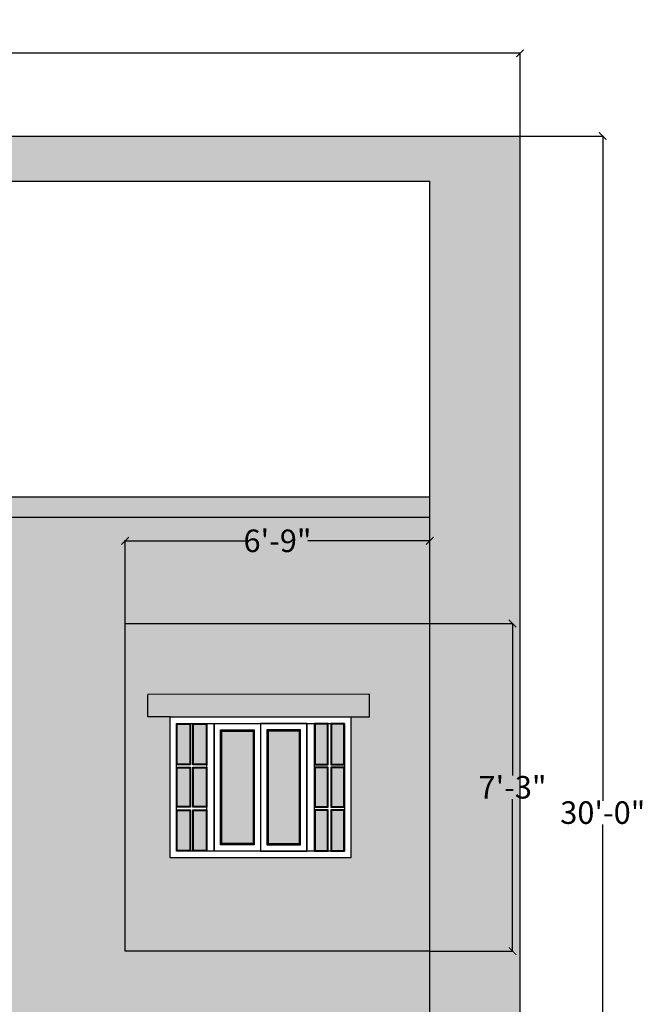
# Model space of a CAD drawing. Units: inches. Extents: x 528 to 2620, y -1066 to 798.
# Tile 41 of 41: x 2453 to 2620, y -891 to -629. Entities that reach past the tile are written whole.
import ezdxf

# ---------------------------------------------------------------- set-up
doc = ezdxf.new("R2010")
doc.units = ezdxf.units.IN
doc.header["$MEASUREMENT"] = 0
for name, color, linetype, lineweight in [('A-ANNO-DIMS', 2, 'Continuous', 18), ('A-ELEV', 7, 'Continuous', 25), ('A-ELEV-PATT', 8, 'Continuous', 13)]:
    doc.layers.add(name, color=color, linetype=linetype, lineweight=lineweight)
doc.styles.get("Standard").update_dxf_attribs({"font": 'arial.ttf'})
doc.dimstyles.get("Standard").update_dxf_attribs({"dimtxt": 6, "dimasz": 2, "dimexe": 0.18, "dimexo": 0.0625, "dimgap": 0.09, "dimtad": 0, "dimtih": 1, "dimtoh": 1, "dimdec": 1, "dimzin": 0, "dimdsep": 46, "dimlunit": 3, "dimtxsty": 'Standard', "dimblk": 'ARCHTICK', "dimcen": 0.09, "dimadec": 0, "dimazin": 0, "dimtfac": 1, "dimtdec": 1, "dimtofl": 0, "dimtmove": 0, "dimatfit": 3, "dimfxl": 1, "dimtolj": 1, "dimtzin": 0, "dimarcsym": 0})

# ---------------------------------------------------------------- blocks, each defined once
blk = doc.blocks.new('ww')
at = {"color": 0, "linetype": 'ByBlock'}
for p, q in [((30.67, -16.13), (126.65, -16.13)), ((30.67, -91.08), (30.67, -16.13)), ((34.01, -19.6), (123.32, -19.6)), ((34.01, -87.61), (34.01, -19.6)), ((34.01, -19.6), (49.87, -19.6)), ((34.01, -87.61), (34.01, -19.6)), ((50.03, -87.61), (50.03, -19.6)), ((54.03, -19.6), (54.03, -87.61)), ((103.29, -19.6), (103.29, -87.61)), ((107.29, -87.61), (107.29, -19.6)), ((123.32, -19.6), (123.32, -87.61)), ((126.65, -16.13), (126.65, -91.08)), ((123.32, -87.61), (34.01, -87.61)), ((126.65, -91.08), (30.67, -91.08))]:
    blk.add_line(p, q, dxfattribs=at)
at = {"color": 0, "linetype": 'ByBlock', "ltscale": 25}
for p, q in [((34.01, -41.58), (34.01, -19.6)), ((34.01, -19.6), (41.35, -19.6)), ((34.34, -41.23), (34.34, -19.95)), ((34.34, -19.95), (41.02, -19.95)), ((41.02, -19.95), (41.02, -41.23)), ((41.35, -19.6), (41.35, -41.58)), ((42.69, -41.58), (42.69, -19.6)), ((42.69, -19.6), (50.03, -19.6)), ((43.02, -41.23), (43.02, -19.95)), ((43.02, -19.95), (49.7, -19.95)), ((49.7, -19.95), (49.7, -41.23)), ((50.03, -19.6), (50.03, -41.58)), ((54.03, -87.61), (54.03, -19.6)), ((54.03, -19.6), (78.66, -19.6)), ((103.29, -19.6), (78.66, -19.6)), ((78.66, -19.6), (78.66, -87.61)), ((78.66, -19.6), (78.66, -87.61)), ((103.29, -87.61), (103.29, -19.6)), ((107.29, -19.6), (107.29, -41.58)), ((114.63, -19.6), (107.29, -19.6)), ((107.62, -19.95), (107.62, -41.23)), ((114.3, -19.95), (107.62, -19.95)), ((114.3, -41.23), (114.3, -19.95)), ((114.63, -41.58), (114.63, -19.6)), ((115.97, -19.6), (115.97, -41.58)), ((123.32, -19.6), (115.97, -19.6)), ((116.3, -19.95), (116.3, -41.23)), ((122.98, -19.95), (116.3, -19.95)), ((122.98, -41.23), (122.98, -19.95)), ((123.32, -41.58), (123.32, -19.6)), ((57.37, -84.14), (57.37, -23.07)), ((57.37, -23.07), (75.33, -23.07)), ((57.7, -83.8), (57.7, -23.42)), ((57.7, -23.42), (74.99, -23.42)), ((58.03, -83.45), (58.03, -23.77)), ((58.03, -23.77), (74.66, -23.77)), ((74.66, -23.77), (74.66, -83.45)), ((74.99, -23.42), (74.99, -83.8)), ((75.33, -23.07), (75.33, -84.14)), ((99.96, -23.07), (81.99, -23.07)), ((81.99, -23.07), (81.99, -84.14)), ((99.62, -23.42), (82.33, -23.42)), ((82.33, -23.42), (82.33, -83.8)), ((99.29, -23.77), (82.66, -23.77)), ((82.66, -23.77), (82.66, -83.45)), ((99.29, -83.45), (99.29, -23.77)), ((99.62, -83.8), (99.62, -23.42)), ((99.96, -84.14), (99.96, -23.07)), ((41.35, -41.58), (34.01, -41.58)), ((41.02, -41.23), (34.34, -41.23)), ((50.03, -41.58), (42.69, -41.58)), ((49.7, -41.23), (43.02, -41.23)), ((107.29, -41.58), (114.63, -41.58)), ((107.62, -41.23), (114.3, -41.23)), ((115.97, -41.58), (123.32, -41.58)), ((116.3, -41.23), (122.98, -41.23)), ((34.01, -64.25), (34.01, -42.97)), ((34.01, -42.97), (41.35, -42.97)), ((34.34, -63.9), (34.34, -43.31)), ((34.34, -43.31), (41.02, -43.31)), ((41.02, -43.31), (41.02, -63.9)), ((41.35, -42.97), (41.35, -64.25)), ((42.69, -64.25), (42.69, -42.97)), ((42.69, -42.97), (50.03, -42.97)), ((43.02, -63.9), (43.02, -43.31)), ((43.02, -43.31), (49.7, -43.31)), ((49.7, -43.31), (49.7, -63.9)), ((50.03, -42.97), (50.03, -64.25)), ((107.29, -42.97), (107.29, -64.25)), ((114.63, -42.97), (107.29, -42.97)), ((107.62, -43.31), (107.62, -63.9)), ((114.3, -43.31), (107.62, -43.31)), ((114.3, -63.9), (114.3, -43.31)), ((114.63, -64.25), (114.63, -42.97)), ((115.97, -42.97), (115.97, -64.25)), ((123.32, -42.97), (115.97, -42.97)), ((116.3, -43.31), (116.3, -63.9)), ((122.98, -43.31), (116.3, -43.31)), ((122.98, -63.9), (122.98, -43.31)), ((123.32, -64.25), (123.32, -42.97)), ((41.35, -64.25), (34.01, -64.25)), ((34.01, -87.61), (34.01, -65.64)), ((34.01, -65.64), (41.35, -65.64)), ((41.02, -63.9), (34.34, -63.9)), ((34.34, -87.27), (34.34, -65.98)), ((34.34, -65.98), (41.02, -65.98)), ((41.02, -65.98), (41.02, -87.27)), ((41.35, -65.64), (41.35, -87.61)), ((50.03, -64.25), (42.69, -64.25)), ((42.69, -87.61), (42.69, -65.64)), ((42.69, -65.64), (50.03, -65.64)), ((49.7, -63.9), (43.02, -63.9)), ((43.02, -87.27), (43.02, -65.98)), ((43.02, -65.98), (49.7, -65.98)), ((49.7, -65.98), (49.7, -87.27)), ((50.03, -65.64), (50.03, -87.61)), ((107.29, -64.25), (114.63, -64.25)), ((107.29, -65.64), (107.29, -87.61)), ((114.63, -65.64), (107.29, -65.64)), ((107.62, -63.9), (114.3, -63.9)), ((107.62, -65.98), (107.62, -87.27)), ((114.3, -65.98), (107.62, -65.98)), ((114.3, -87.27), (114.3, -65.98)), ((114.63, -87.61), (114.63, -65.64)), ((115.97, -64.25), (123.32, -64.25)), ((115.97, -65.64), (115.97, -87.61)), ((123.32, -65.64), (115.97, -65.64)), ((116.3, -63.9), (122.98, -63.9)), ((116.3, -65.98), (116.3, -87.27)), ((122.98, -65.98), (116.3, -65.98)), ((122.98, -87.27), (122.98, -65.98)), ((123.32, -87.61), (123.32, -65.64)), ((74.99, -83.8), (57.7, -83.8)), ((74.66, -83.45), (58.03, -83.45)), ((82.33, -83.8), (99.62, -83.8)), ((82.66, -83.45), (99.29, -83.45)), ((41.35, -87.61), (34.01, -87.61)), ((41.02, -87.27), (34.34, -87.27)), ((50.03, -87.61), (42.69, -87.61)), ((49.7, -87.27), (43.02, -87.27)), ((78.66, -87.61), (54.03, -87.61)), ((75.33, -84.14), (57.37, -84.14)), ((78.66, -87.61), (103.29, -87.61)), ((81.99, -84.14), (99.96, -84.14)), ((107.29, -87.61), (114.63, -87.61)), ((107.62, -87.27), (114.3, -87.27)), ((115.97, -87.61), (123.32, -87.61)), ((116.3, -87.27), (122.98, -87.27))]:
    blk.add_line(p, q, dxfattribs=at)
blk = doc.blocks.new('_ArchTick')
at = {"color": 0, "linetype": 'ByBlock', "const_width": 0.15}
blk.add_lwpolyline([(-0.5, -0.5), (0.5, 0.5)], dxfattribs=at)
blk = doc.blocks.new('*D69')
at = {"layer": 'A-ANNO-DIMS', "color": 0, "lineweight": -2, "transparency": 16777216}
for p, q in [((2586.61, -660.15), (2608.73, -660.15)), ((2608.55, -660.15), (2608.55, -836.99)), ((2608.55, -1020.15), (2608.55, -843.3)), ((2586.61, -1020.15), (2608.73, -1020.15))]:
    blk.add_line(p, q, dxfattribs=at)
at = {"layer": 'Defpoints', "color": 0, "transparency": 16777216}
for p in [(2586.55, -660.15), (2608.55, -660.15), (2586.55, -1020.15)]:
    blk.add_point(p, dxfattribs=at)
at = {"layer": 'A-ANNO-DIMS', "color": 0, "lineweight": -2, "transparency": 16777216, "xscale": 2, "yscale": 2, "zscale": 2}
for p, rotation in [((2608.55, -660.15), 90), ((2608.55, -1020.15), 270)]:
    blk.add_blockref('_ArchTick', p, dxfattribs=dict(at, rotation=rotation))
at = {"layer": 'A-ANNO-DIMS', "color": 0, "transparency": 16777216, "insert": (2608.55, -840.15), "char_height": 6, "attachment_point": 5}
blk.add_mtext('\\A1;30\'-0"', dxfattribs=at)
blk = doc.blocks.new('*D70')
at = {"layer": 'A-ANNO-DIMS', "color": 0, "lineweight": -2, "transparency": 16777216}
for p, q in [((2266.05, -852.09), (2266.05, -637.97)), ((2266.05, -638.15), (2408.86, -638.15)), ((2586.55, -638.15), (2443.73, -638.15)), ((2586.55, -660.09), (2586.55, -637.97))]:
    blk.add_line(p, q, dxfattribs=at)
at = {"layer": 'Defpoints', "color": 0, "transparency": 16777216}
for p in [(2586.55, -638.15), (2586.55, -660.15), (2266.05, -852.15)]:
    blk.add_point(p, dxfattribs=at)
at = {"layer": 'A-ANNO-DIMS', "color": 0, "lineweight": -2, "transparency": 16777216, "xscale": 2, "yscale": 2, "zscale": 2, "rotation": 180}
blk.add_blockref('_ArchTick', (2266.05, -638.15), dxfattribs=at)
at = {"layer": 'A-ANNO-DIMS', "color": 0, "lineweight": -2, "transparency": 16777216, "xscale": 2, "yscale": 2, "zscale": 2}
blk.add_blockref('_ArchTick', (2586.55, -638.15), dxfattribs=at)
at = {"layer": 'A-ANNO-DIMS', "color": 0, "transparency": 16777216, "insert": (2426.3, -638.15), "char_height": 6, "attachment_point": 5}
blk.add_mtext('\\A1;26\'-8 1/2"', dxfattribs=at)
blk = doc.blocks.new('*D89')
at = {"layer": 'A-ANNO-DIMS', "color": 0, "lineweight": -2, "transparency": 16777216}
for p, q in [((2481.55, -789.78), (2481.55, -767.66)), ((2481.55, -767.84), (2513.96, -767.84)), ((2562.55, -767.84), (2530.13, -767.84)), ((2562.55, -789.78), (2562.55, -767.66))]:
    blk.add_line(p, q, dxfattribs=at)
at = {"layer": 'Defpoints', "color": 0, "transparency": 16777216}
for p in [(2562.55, -767.84), (2481.55, -789.84), (2562.55, -789.84)]:
    blk.add_point(p, dxfattribs=at)
at = {"layer": 'A-ANNO-DIMS', "color": 0, "lineweight": -2, "transparency": 16777216, "xscale": 2, "yscale": 2, "zscale": 2, "rotation": 180}
blk.add_blockref('_ArchTick', (2481.55, -767.84), dxfattribs=at)
at = {"layer": 'A-ANNO-DIMS', "color": 0, "lineweight": -2, "transparency": 16777216, "xscale": 2, "yscale": 2, "zscale": 2}
blk.add_blockref('_ArchTick', (2562.55, -767.84), dxfattribs=at)
at = {"layer": 'A-ANNO-DIMS', "color": 0, "transparency": 16777216, "insert": (2522.05, -767.84), "char_height": 6, "attachment_point": 5}
blk.add_mtext('\\A1;6\'-9"', dxfattribs=at)
blk = doc.blocks.new('*D92')
at = {"layer": 'A-ANNO-DIMS', "color": 0, "lineweight": -2, "transparency": 16777216}
for p, q in [((2562.61, -789.84), (2584.73, -789.84)), ((2584.55, -789.84), (2584.55, -830.25)), ((2584.55, -876.97), (2584.55, -836.56)), ((2562.61, -876.97), (2584.73, -876.97))]:
    blk.add_line(p, q, dxfattribs=at)
at = {"layer": 'Defpoints', "color": 0, "transparency": 16777216}
for p in [(2562.55, -789.84), (2562.55, -876.97), (2584.55, -876.97)]:
    blk.add_point(p, dxfattribs=at)
at = {"layer": 'A-ANNO-DIMS', "color": 0, "lineweight": -2, "transparency": 16777216, "xscale": 2, "yscale": 2, "zscale": 2}
for p, rotation in [((2584.55, -789.84), 90), ((2584.55, -876.97), 270)]:
    blk.add_blockref('_ArchTick', p, dxfattribs=dict(at, rotation=rotation))
at = {"layer": 'A-ANNO-DIMS', "color": 0, "transparency": 16777216, "insert": (2584.55, -833.41), "char_height": 6, "attachment_point": 5}
blk.add_mtext('\\A1;7\'-3"', dxfattribs=at)

msp = doc.modelspace()

# ---------------------------------------------------------------- hatches: boundary and pattern name
at = {"layer": 'A-ELEV-PATT', "transparency": 33554687}
h = msp.add_hatch(color=256, dxfattribs=at)
h.dxf.hatch_style = 1
h.paths.add_polyline_path([(2586.55, -660.15), (2298.55, -660.15), (2298.55, -720.15), (2310.55, -720.15), (2310.55, -672.15), (2562.55, -672.15), (2562.55, -900.15), (2448.55, -900.15), (2448.55, -912.15), (2586.55, -912.15)])
h = msp.add_hatch(color=256, dxfattribs=at)
h.dxf.hatch_style = 1
h.paths.add_polyline_path([(2562.55, -756.15), (2448.55, -756.15), (2448.55, -761.55), (2562.55, -761.55)])
h = msp.add_hatch(color=256, dxfattribs=at)
h.dxf.hatch_style = 1
h.paths.add_polyline_path([(2586.55, -912.15), (2448.55, -912.15), (2448.55, -940.66), (2547.55, -940.66), (2547.55, -990.15), (2448.55, -990.15), (2448.55, -1020.15), (2586.55, -1020.15)])
h.paths.add_polyline_path([(2481.55, -789.84), (2562.55, -789.84), (2562.55, -761.55), (2448.55, -761.55), (2448.55, -900.15), (2562.55, -900.15), (2562.55, -876.97), (2481.55, -876.97), (2481.55, -833.41)])
h.paths.add_polyline_path([(2412.55, -780.15), (2298.55, -780.15), (2298.55, -852.15), (2322.55, -852.15), (2322.55, -814.66), (2370.55, -814.66), (2370.55, -852.15), (2412.55, -852.15)])
h.paths.add_polyline_path([(2394.55, -940.36), (2442.55, -940.36), (2442.55, -1020.15), (2448.55, -1020.15), (2448.55, -990.15), (2448.55, -912.15), (2310.55, -912.15), (2310.55, -1020.15), (2394.55, -1020.15)])
h.paths.add_polyline_path([(2327.05, -984.15), (2327.05, -946.66), (2375.05, -946.66), (2375.05, -984.15)], flags=16)
h.paths.add_polyline_path([(2328.71, -982.41), (2328.71, -948.4), (2336.65, -948.4), (2336.73, -948.4), (2373.38, -948.4), (2373.38, -982.41), (2369.7, -982.41)], flags=0)
h.paths.add_polyline_path([(2338.73, -982.41), (2338.73, -948.4), (2351.05, -948.4), (2363.36, -948.4), (2363.36, -982.41), (2351.05, -982.41)], flags=0)
h.paths.add_polyline_path([(2340.4, -980.68), (2340.4, -950.13), (2349.38, -950.13), (2349.38, -980.68)], flags=0)
h.paths.add_polyline_path([(2340.73, -980.33), (2340.73, -950.48), (2349.05, -950.48), (2349.05, -980.33)], flags=0)
h.paths.add_polyline_path([(2352.71, -980.68), (2352.71, -950.13), (2361.7, -950.13), (2361.7, -980.68)], flags=0)
h.paths.add_polyline_path([(2353.05, -980.33), (2353.05, -950.48), (2361.36, -950.48), (2361.36, -980.33)], flags=0)
h.paths.add_polyline_path([(2336.73, -982.41), (2333.05, -982.41), (2333.05, -971.42), (2336.73, -971.42), (2336.73, -970.73), (2333.05, -970.73), (2333.05, -960.08), (2336.73, -960.08), (2336.73, -959.39), (2333.05, -959.39), (2333.05, -948.57), (2336.73, -948.57)], flags=0)
h.paths.add_polyline_path([(2333.22, -982.24), (2333.22, -971.6), (2336.73, -971.6), (2336.73, -982.24)], flags=0)
h.paths.add_polyline_path([(2332.39, -982.41), (2328.71, -982.41), (2328.71, -948.4), (2332.39, -948.4), (2332.39, -959.39), (2328.71, -959.39), (2328.71, -960.08), (2332.39, -960.08), (2332.39, -970.73), (2328.71, -970.73), (2328.71, -971.42), (2332.39, -971.42)], flags=0)
h.paths.add_polyline_path([(2332.22, -982.24), (2328.71, -982.24), (2328.71, -971.6), (2332.22, -971.6)], flags=0)
h.paths.add_polyline_path([(2365.36, -982.41), (2365.36, -948.4), (2369.04, -948.4), (2369.04, -959.39), (2365.36, -959.39), (2365.36, -960.08), (2369.04, -960.08), (2369.04, -970.73), (2365.36, -970.73), (2365.36, -971.42), (2369.04, -971.42), (2369.04, -982.41)], flags=0)
h.paths.add_polyline_path([(2369.7, -971.42), (2373.38, -971.42), (2373.38, -982.24), (2369.7, -982.24)], flags=0)
h.paths.add_polyline_path([(2333.22, -970.55), (2333.22, -960.26), (2336.73, -960.26), (2336.73, -970.55)], flags=0)
h.paths.add_polyline_path([(2332.22, -970.55), (2328.71, -970.55), (2328.71, -960.26), (2332.22, -960.26)], flags=0)
h.paths.add_polyline_path([(2369.7, -970.73), (2369.7, -960.08), (2373.38, -960.08), (2373.38, -970.73)], flags=0)
h.paths.add_polyline_path([(2336.56, -959.22), (2336.56, -948.57), (2336.73, -948.4), (2336.73, -959.22)], flags=0)
h.paths.add_polyline_path([(2332.22, -959.22), (2328.71, -959.22), (2328.71, -948.57), (2332.22, -948.57)], flags=0)
h.paths.add_polyline_path([(2369.7, -959.39), (2369.7, -948.4), (2373.38, -948.4), (2373.38, -959.39)], flags=0)
h = msp.add_hatch(color=256, dxfattribs=at)
h.dxf.hatch_style = 1
h.paths.add_polyline_path([(2562.55, -789.84), (2481.55, -789.84), (2481.55, -833.41), (2481.55, -876.97), (2562.55, -876.97)])
h.paths.add_polyline_path([(2541.55, -852.15), (2493.55, -852.15), (2493.55, -814.66), (2487.57, -814.66), (2487.57, -808.71), (2546.5, -808.65), (2546.5, -814.66), (2541.55, -814.66)], flags=16)
h.paths.add_polyline_path([(2539.88, -850.41), (2536.2, -850.41), (2495.21, -850.41), (2495.21, -816.4), (2503.15, -816.4), (2503.23, -816.4), (2539.88, -816.4)], flags=0)
h.paths.add_polyline_path([(2539.88, -838.73), (2536.2, -838.73), (2536.2, -828.08), (2539.88, -828.08)], flags=0)
h.paths.add_polyline_path([(2539.88, -839.42), (2539.88, -850.24), (2536.2, -850.24), (2536.2, -839.42)], flags=0)
h.paths.add_polyline_path([(2539.71, -838.55), (2536.37, -838.55), (2536.37, -828.26), (2539.71, -828.26)], flags=0)
h.paths.add_polyline_path([(2535.54, -838.73), (2531.86, -838.73), (2531.86, -839.42), (2535.54, -839.42), (2535.54, -850.41), (2531.86, -850.41), (2531.86, -816.4), (2535.54, -816.4), (2535.54, -827.39), (2531.86, -827.39), (2531.86, -828.08), (2535.54, -828.08)], flags=0)
h.paths.add_polyline_path([(2535.37, -838.55), (2531.86, -838.55), (2531.86, -828.26), (2535.37, -828.26)], flags=0)
h.paths.add_polyline_path([(2535.37, -839.6), (2535.37, -850.24), (2531.86, -850.24), (2531.86, -839.6)], flags=0)
h.paths.add_polyline_path([(2539.88, -827.39), (2536.2, -827.39), (2536.2, -816.4), (2539.88, -816.4)], flags=0)
h.paths.add_polyline_path([(2539.71, -827.22), (2536.37, -827.22), (2536.37, -816.57), (2539.71, -816.57)], flags=0)
h.paths.add_polyline_path([(2535.37, -827.22), (2531.86, -827.22), (2531.86, -816.57), (2535.37, -816.57)], flags=0)
h.paths.add_polyline_path([(2529.86, -850.41), (2517.55, -850.41), (2505.23, -850.41), (2505.23, -816.4), (2517.55, -816.4), (2529.86, -816.4)], flags=0)
h.paths.add_polyline_path([(2528.2, -848.68), (2519.21, -848.68), (2519.21, -818.13), (2528.2, -818.13)], flags=0)
h.paths.add_polyline_path([(2528.03, -848.5), (2519.38, -848.5), (2519.38, -818.31), (2528.03, -818.31)], flags=0)
h.paths.add_polyline_path([(2527.86, -848.33), (2519.55, -848.33), (2519.55, -818.48), (2527.86, -818.48)], flags=0)
h.paths.add_polyline_path([(2515.88, -848.68), (2506.9, -848.68), (2506.9, -818.13), (2515.88, -818.13)], flags=0)
h.paths.add_polyline_path([(2515.71, -848.5), (2507.06, -848.5), (2507.06, -818.31), (2515.71, -818.31)], flags=0)
h.paths.add_polyline_path([(2515.55, -848.33), (2507.23, -848.33), (2507.23, -818.48), (2515.55, -818.48)], flags=0)
h.paths.add_polyline_path([(2503.23, -850.41), (2499.55, -850.41), (2499.55, -839.42), (2503.23, -839.42), (2503.23, -838.73), (2499.55, -838.73), (2499.55, -828.08), (2503.23, -828.08), (2503.23, -827.39), (2499.55, -827.39), (2499.55, -816.57), (2503.23, -816.57)], flags=0)
h.paths.add_polyline_path([(2503.23, -838.55), (2499.72, -838.55), (2499.72, -828.26), (2503.23, -828.26)], flags=0)
h.paths.add_polyline_path([(2503.23, -850.24), (2499.72, -850.24), (2499.72, -839.6), (2503.23, -839.6)], flags=0)
h.paths.add_polyline_path([(2503.06, -816.57), (2503.23, -816.4), (2503.23, -827.22), (2503.06, -827.22)], flags=0)
h.paths.add_polyline_path([(2498.89, -838.73), (2495.21, -838.73), (2495.21, -839.42), (2498.89, -839.42), (2498.89, -850.41), (2495.21, -850.41), (2495.21, -816.4), (2498.89, -816.4), (2498.89, -827.39), (2495.21, -827.39), (2495.21, -828.08), (2498.89, -828.08)], flags=0)
h.paths.add_polyline_path([(2498.72, -838.55), (2495.21, -838.55), (2495.21, -828.26), (2498.72, -828.26)], flags=0)
h.paths.add_polyline_path([(2498.72, -839.6), (2498.72, -850.24), (2495.21, -850.24), (2495.21, -839.6)], flags=0)
h.paths.add_polyline_path([(2498.72, -827.22), (2495.21, -827.22), (2495.21, -816.57), (2498.72, -816.57)], flags=0)
h.paths.add_polyline_path([(2547.55, -940.66), (2448.55, -940.66), (2448.55, -990.15), (2547.55, -990.15)])
h.paths.add_polyline_path([(2493.55, -946.66), (2541.55, -946.66), (2541.55, -984.15), (2493.55, -984.15)], flags=16)
h.paths.add_polyline_path([(2495.21, -948.4), (2503.15, -948.4), (2503.23, -948.4), (2539.88, -948.4), (2539.88, -982.41), (2536.2, -982.41), (2495.21, -982.41)], flags=0)
h.paths.add_polyline_path([(2495.21, -948.4), (2498.89, -948.4), (2498.89, -959.39), (2495.21, -959.39), (2495.21, -960.08), (2498.89, -960.08), (2498.89, -970.73), (2495.21, -970.73), (2495.21, -971.42), (2498.89, -971.42), (2498.89, -982.41), (2495.21, -982.41)], flags=0)
h.paths.add_polyline_path([(2498.72, -960.26), (2498.72, -970.55), (2495.21, -970.55), (2495.21, -960.26)], flags=0)
h.paths.add_polyline_path([(2498.72, -971.6), (2498.72, -982.24), (2495.21, -982.24), (2495.21, -971.6)], flags=0)
h.paths.add_polyline_path([(2499.55, -948.57), (2503.23, -948.57), (2503.23, -982.41), (2499.55, -982.41), (2499.55, -971.42), (2503.23, -971.42), (2503.23, -970.73), (2499.55, -970.73), (2499.55, -960.08), (2503.23, -960.08), (2503.23, -959.39), (2499.55, -959.39)], flags=0)
h.paths.add_polyline_path([(2503.06, -959.22), (2503.06, -948.57), (2503.23, -948.4), (2503.23, -959.22)], flags=0)
h.paths.add_polyline_path([(2499.72, -960.26), (2503.23, -960.26), (2503.23, -970.55), (2499.72, -970.55)], flags=0)
h.paths.add_polyline_path([(2499.72, -971.6), (2503.23, -971.6), (2503.23, -982.24), (2499.72, -982.24)], flags=0)
h.paths.add_polyline_path([(2505.23, -948.4), (2517.55, -948.4), (2529.86, -948.4), (2529.86, -982.41), (2517.55, -982.41), (2505.23, -982.41)], flags=0)
h.paths.add_polyline_path([(2506.9, -950.13), (2515.88, -950.13), (2515.88, -980.68), (2506.9, -980.68)], flags=0)
h.paths.add_polyline_path([(2507.23, -950.48), (2515.55, -950.48), (2515.55, -980.33), (2507.23, -980.33)], flags=0)
h.paths.add_polyline_path([(2519.21, -950.13), (2528.2, -950.13), (2528.2, -980.68), (2519.21, -980.68)], flags=0)
h.paths.add_polyline_path([(2519.55, -950.48), (2527.86, -950.48), (2527.86, -980.33), (2519.55, -980.33)], flags=0)
h.paths.add_polyline_path([(2531.86, -948.4), (2535.54, -948.4), (2535.54, -959.39), (2531.86, -959.39), (2531.86, -960.08), (2535.54, -960.08), (2535.54, -970.73), (2531.86, -970.73), (2531.86, -971.42), (2535.54, -971.42), (2535.54, -982.41), (2531.86, -982.41)], flags=0)
h.paths.add_polyline_path([(2535.37, -960.26), (2535.37, -970.55), (2531.86, -970.55), (2531.86, -960.26)], flags=0)
h.paths.add_polyline_path([(2535.37, -971.6), (2535.37, -982.24), (2531.86, -982.24), (2531.86, -971.6)], flags=0)
h.paths.add_polyline_path([(2536.2, -948.4), (2539.88, -948.4), (2539.88, -959.39), (2536.2, -959.39)], flags=0)
h.paths.add_polyline_path([(2536.2, -960.08), (2539.88, -960.08), (2539.88, -970.73), (2536.2, -970.73)], flags=0)
h.paths.add_polyline_path([(2536.2, -971.42), (2539.88, -971.42), (2539.88, -982.24), (2536.2, -982.24)], flags=0)
h = msp.add_hatch(color=256, dxfattribs=at)
h.dxf.hatch_style = 1
h.paths.add_polyline_path([(2546.5, -808.65), (2487.57, -808.71), (2487.57, -814.66), (2493.55, -814.66), (2541.55, -814.66), (2546.5, -814.66)])
h = msp.add_hatch(color=256, dxfattribs=at)
h.dxf.hatch_style = 1
h.paths.add_polyline_path([(2527.86, -818.48), (2519.55, -818.48), (2519.55, -848.33), (2527.86, -848.33)])
h.paths.add_polyline_path([(2515.55, -818.48), (2507.23, -818.48), (2507.23, -848.33), (2515.55, -848.33)])
h.paths.add_polyline_path([(2498.72, -816.57), (2495.38, -816.57), (2495.38, -827.22), (2498.72, -827.22)])
h.paths.add_polyline_path([(2503.06, -816.57), (2499.72, -816.57), (2499.72, -827.22), (2503.06, -827.22)])
h.paths.add_polyline_path([(2498.72, -828.26), (2495.38, -828.26), (2495.38, -838.55), (2498.72, -838.55)])
h.paths.add_polyline_path([(2503.06, -828.26), (2499.72, -828.26), (2499.72, -838.55), (2503.06, -838.55)])
h.paths.add_polyline_path([(2498.72, -839.6), (2495.38, -839.6), (2495.38, -850.24), (2498.72, -850.24)])
h.paths.add_polyline_path([(2503.06, -839.6), (2499.72, -839.6), (2499.72, -850.24), (2503.06, -850.24)])
h.paths.add_polyline_path([(2535.37, -839.6), (2532.03, -839.6), (2532.03, -850.24), (2535.37, -850.24)])
h.paths.add_polyline_path([(2539.71, -839.6), (2536.37, -839.6), (2536.37, -850.24), (2539.71, -850.24)])
h.paths.add_polyline_path([(2535.37, -828.26), (2532.03, -828.26), (2532.03, -838.55), (2535.37, -838.55)])
h.paths.add_polyline_path([(2539.71, -828.26), (2536.37, -828.26), (2536.37, -838.55), (2539.71, -838.55)])
h.paths.add_polyline_path([(2535.37, -816.57), (2532.03, -816.57), (2532.03, -827.22), (2535.37, -827.22)])
h.paths.add_polyline_path([(2356.86, -818.48), (2348.55, -818.48), (2348.55, -848.33), (2356.86, -848.33)])
h.paths.add_polyline_path([(2344.55, -818.48), (2336.23, -818.48), (2336.23, -848.33), (2344.55, -848.33)])
h.paths.add_polyline_path([(2327.72, -816.57), (2324.38, -816.57), (2324.38, -827.22), (2327.72, -827.22)])
h.paths.add_polyline_path([(2332.06, -816.57), (2328.72, -816.57), (2328.72, -827.22), (2332.06, -827.22)])
h.paths.add_polyline_path([(2327.72, -828.26), (2324.38, -828.26), (2324.38, -838.55), (2327.72, -838.55)])
h.paths.add_polyline_path([(2332.06, -828.26), (2328.72, -828.26), (2328.72, -838.55), (2332.06, -838.55)])
h.paths.add_polyline_path([(2327.72, -839.6), (2324.38, -839.6), (2324.38, -850.24), (2327.72, -850.24)])
h.paths.add_polyline_path([(2332.06, -839.6), (2328.72, -839.6), (2328.72, -850.24), (2332.06, -850.24)])
h.paths.add_polyline_path([(2368.71, -839.6), (2365.37, -839.6), (2365.37, -850.24), (2368.71, -850.24)])
h.paths.add_polyline_path([(2364.37, -839.6), (2361.03, -839.6), (2361.03, -850.24), (2364.37, -850.24)])
h.paths.add_polyline_path([(2364.37, -828.26), (2361.03, -828.26), (2361.03, -838.55), (2364.37, -838.55)])
h.paths.add_polyline_path([(2368.71, -828.26), (2365.37, -828.26), (2365.37, -838.55), (2368.71, -838.55)])
h.paths.add_polyline_path([(2364.37, -816.57), (2361.03, -816.57), (2361.03, -827.22), (2364.37, -827.22)])
h.paths.add_polyline_path([(2368.71, -816.57), (2365.37, -816.57), (2365.37, -827.22), (2368.71, -827.22)])
h.paths.add_polyline_path([(2361.36, -950.48), (2353.05, -950.48), (2353.05, -980.33), (2361.36, -980.33)])
h.paths.add_polyline_path([(2349.05, -950.48), (2340.73, -950.48), (2340.73, -980.33), (2349.05, -980.33)])
h.paths.add_polyline_path([(2336.56, -971.6), (2333.22, -971.6), (2333.22, -982.24), (2336.56, -982.24)])
h.paths.add_polyline_path([(2332.22, -971.6), (2328.88, -971.6), (2328.88, -982.24), (2332.22, -982.24)])
h.paths.add_polyline_path([(2336.56, -960.26), (2333.22, -960.26), (2333.22, -970.55), (2336.56, -970.55)])
h.paths.add_polyline_path([(2332.22, -960.26), (2328.88, -960.26), (2328.88, -970.55), (2332.22, -970.55)])
h.paths.add_polyline_path([(2332.22, -948.57), (2328.88, -948.57), (2328.88, -959.22), (2332.22, -959.22)])
h.paths.add_polyline_path([(2336.56, -948.57), (2333.22, -948.57), (2333.22, -959.22), (2336.56, -959.22)])
h.paths.add_polyline_path([(2368.87, -971.6), (2365.53, -971.6), (2365.53, -982.24), (2368.87, -982.24)])
h.paths.add_polyline_path([(2373.21, -971.6), (2369.87, -971.6), (2369.87, -982.24), (2373.21, -982.24)])
h.paths.add_polyline_path([(2373.21, -960.26), (2369.87, -960.26), (2369.87, -970.55), (2373.21, -970.55)])
h.paths.add_polyline_path([(2368.87, -960.26), (2365.53, -960.26), (2365.53, -970.55), (2368.87, -970.55)])
h.paths.add_polyline_path([(2368.87, -948.57), (2365.53, -948.57), (2365.53, -959.22), (2368.87, -959.22)])
h.paths.add_polyline_path([(2373.21, -948.57), (2369.87, -948.57), (2369.87, -959.22), (2373.21, -959.22)])
h.paths.add_polyline_path([(2527.86, -950.48), (2519.55, -950.48), (2519.55, -980.33), (2527.86, -980.33)])
h.paths.add_polyline_path([(2515.55, -950.48), (2507.23, -950.48), (2507.23, -980.33), (2515.55, -980.33)])
h.paths.add_polyline_path([(2539.71, -971.6), (2536.37, -971.6), (2536.37, -982.24), (2539.71, -982.24)])
h.paths.add_polyline_path([(2535.37, -971.6), (2532.03, -971.6), (2532.03, -982.24), (2535.37, -982.24)])
h.paths.add_polyline_path([(2535.37, -960.26), (2532.03, -960.26), (2532.03, -970.55), (2535.37, -970.55)])
h.paths.add_polyline_path([(2539.71, -960.26), (2536.37, -960.26), (2536.37, -970.55), (2539.71, -970.55)])
h.paths.add_polyline_path([(2535.37, -948.57), (2532.03, -948.57), (2532.03, -959.22), (2535.37, -959.22)])
h.paths.add_polyline_path([(2539.71, -948.57), (2536.37, -948.57), (2536.37, -959.22), (2539.71, -959.22)])
h.paths.add_polyline_path([(2498.72, -971.6), (2495.38, -971.6), (2495.38, -982.24), (2498.72, -982.24)])
h.paths.add_polyline_path([(2503.06, -971.6), (2499.72, -971.6), (2499.72, -982.24), (2503.06, -982.24)])
h.paths.add_polyline_path([(2498.72, -960.26), (2495.38, -960.26), (2495.38, -970.55), (2498.72, -970.55)])
h.paths.add_polyline_path([(2503.06, -960.26), (2499.72, -960.26), (2499.72, -970.55), (2503.06, -970.55)])
h.paths.add_polyline_path([(2498.72, -948.57), (2495.38, -948.57), (2495.38, -959.22), (2498.72, -959.22)])
h.paths.add_polyline_path([(2503.06, -948.57), (2499.72, -948.57), (2499.72, -959.22), (2503.06, -959.22)])
h = msp.add_hatch(color=256, dxfattribs=at)
h.dxf.hatch_style = 1
h.paths.add_polyline_path([(2539.71, -816.57), (2536.37, -816.57), (2536.37, -827.22), (2539.71, -827.22)])

# ---------------------------------------------------------------- linework, layer by layer
at = {"layer": 'A-ELEV'}
for p, q in [((2298.55, -660.15), (2586.55, -660.15)), ((2586.55, -1020.15), (2586.55, -660.15)), ((2310.55, -672.15), (2562.55, -672.15)), ((2562.55, -900.15), (2562.55, -672.15)), ((2270.55, -756.15), (2562.55, -756.15)), ((2448.55, -761.55), (2562.55, -761.55)), ((2546.5, -808.65), (2487.57, -808.71)), ((2487.57, -814.66), (2487.57, -808.71)), ((2546.5, -814.66), (2546.5, -808.65)), ((2493.55, -814.66), (2487.57, -814.66)), ((2541.55, -814.66), (2546.5, -814.66))]:
    msp.add_line(p, q, dxfattribs=at)
msp.add_lwpolyline([(2562.55, -876.97), (2481.55, -876.97), (2481.55, -833.41), (2481.55, -789.84), (2562.55, -789.84)], dxfattribs=at)

# ---------------------------------------------------------------- block references
at = {"layer": 'A-ELEV', "xscale": 0.5001250312578946, "yscale": 0.5001250312578946, "zscale": 0.5001250312578946}
msp.add_blockref('ww', (2478.21, -806.6), dxfattribs=at)

# ---------------------------------------------------------------- dimensions: what is measured, and where the dimension line sits
at = {"layer": 'A-ANNO-DIMS'}
for base, p1, p2, picture, middle in [((2586.55, -638.15), (2266.05, -852.15), (2586.55, -660.15), '*D70', (2426.3, -638.15)), ((2562.55, -767.84), (2481.55, -789.84), (2562.55, -789.84), '*D89', (2522.05, -767.84))]:
    dim = msp.add_linear_dim(base=base, p1=p1, p2=p2, dimstyle='Standard', override={"dimdec": 1, "dimlfac": 1, "dimrnd": 0, "dimzin": 1, "dimdsep": 46, "dimlunit": 4, "dimfrac": 2}, dxfattribs=at)
    dim.commit()
    dim.dimension.update_dxf_attribs({"geometry": picture, "text_midpoint": middle})
for base, p1, p2, angle, picture, middle in [((2608.55, -660.15), (2586.55, -1020.15), (2586.55, -660.15), 90, '*D69', (2608.55, -840.15)), ((2584.55, -876.97), (2562.55, -789.84), (2562.55, -876.97), 270, '*D92', (2584.55, -833.41))]:
    dim = msp.add_linear_dim(base=base, p1=p1, p2=p2, angle=angle, dimstyle='Standard', override={"dimdec": 1, "dimlfac": 1, "dimrnd": 0, "dimzin": 1, "dimdsep": 46, "dimlunit": 4, "dimfrac": 2}, dxfattribs=at)
    dim.commit()
    dim.dimension.update_dxf_attribs({"geometry": picture, "text_midpoint": middle})

doc.saveas('drawing.dxf')
